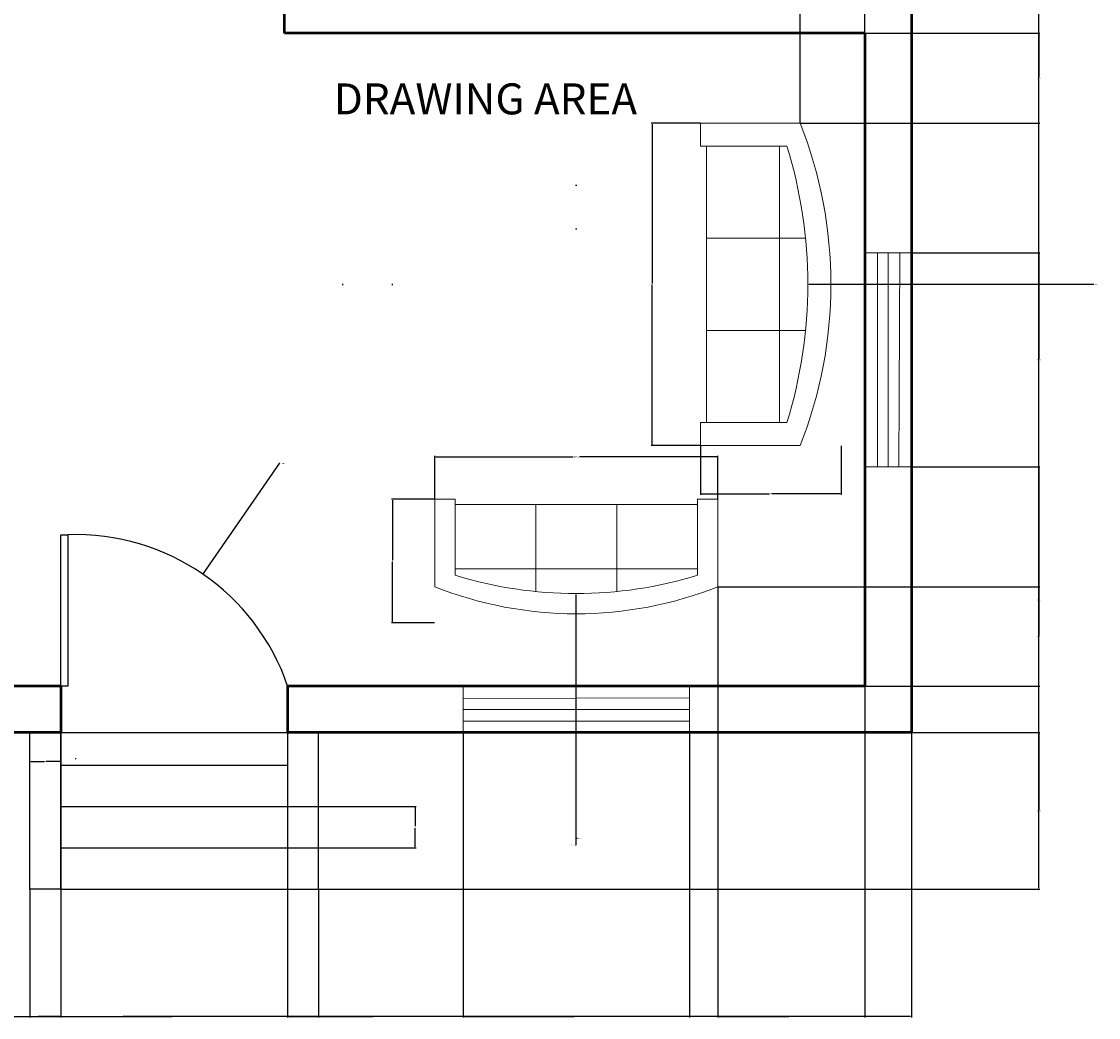
# Model space of a CAD drawing. Units: inches. Extents: x 1926 to 2293, y 1738 to 2280.
# Tile 2 of 6: x 2084 to 2293, y 1738 to 1931. Entities that reach past the tile are written whole.
import ezdxf

# ---------------------------------------------------------------- set-up
doc = ezdxf.new("R2010")
doc.units = ezdxf.units.IN
for name, color, linetype, lineweight in [('A-ANNO-DIMS', 2, 'Continuous', 18), ('A-AREA-IDEN', 7, 'Continuous', 25), ('A-DOOR', 3, 'Continuous', 25), ('A-FLOR-STRS', 7, 'Continuous', 25), ('A-FURN', 8, 'Continuous', 18), ('A-GLAZ', 4, 'Continuous', 18), ('A-WALL', 7, 'Continuous', 50)]:
    doc.layers.add(name, color=color, linetype=linetype, lineweight=lineweight)
doc.styles.get("Standard").update_dxf_attribs({"font": 'arial.ttf'})
doc.dimstyles.get("Standard").update_dxf_attribs({"dimtxt": 0.18, "dimasz": 0.18, "dimexe": 0.18, "dimexo": 0.0625, "dimgap": 0.09, "dimtad": 0, "dimtih": 1, "dimtoh": 1, "dimdec": 4, "dimzin": 0, "dimdsep": 46, "dimtxsty": 'Standard', "dimcen": 0.09, "dimadec": 0, "dimazin": 0, "dimtfac": 1, "dimtdec": 4, "dimtofl": 0, "dimtmove": 0, "dimatfit": 3, "dimfxl": 1, "dimtolj": 1, "dimtzin": 0, "dimarcsym": 0})

# ---------------------------------------------------------------- blocks, each defined once
blk = doc.blocks.new('Sofa - Roundback 7 ft.')
for p, q in [((-12.00002, -32.4421), (-12.00003, -6.5971)), ((11.99997, -32.4421), (11.99998, -6.5971)), ((-36.000027, -34), (-36.000027, -11.4696)), ((-35.999844, -13.3819), (35.9998, -13.3819)), ((35.99998, -34), (35.99998, -11.4696)), ((-36.000027, -32.4421), (35.99998, -32.4421))]:
    blk.add_line(p, q)
for points in [[(-36.000027, -34), (-42.000027, -34), (-42.000027, -8)], [(41.99998, -8), (41.99998, -34), (35.99998, -34)]]:
    blk.add_lwpolyline(points)
for centre, radius, start, end in [((0, -114.25), 114.25, 68.43141, 111.5686), ((-0.00001, -127.1968), 121.1968, 72.72033, 107.2797)]:
    blk.add_arc(centre, radius, start, end)
blk = doc.blocks.new('*D8')
at = {"layer": 'A-ANNO-DIMS', "color": 0, "lineweight": -2, "transparency": 16777216}
for p, q in [((2215.82, 1911.23), (2206.33, 1911.23)), ((2206.51, 1911.05), (2206.51, 1880.18)), ((2206.51, 1848.95), (2206.51, 1879.82)), ((2215.82, 1848.77), (2206.33, 1848.77))]:
    blk.add_line(p, q, dxfattribs=at)
at = {"layer": 'A-ANNO-DIMS', "color": 0, "transparency": 16777216}
for points in [[(2206.48, 1911.05), (2206.54, 1911.05), (2206.51, 1911.23)], [(2206.48, 1848.95), (2206.54, 1848.95), (2206.51, 1848.77)]]:
    blk.add_solid(points, dxfattribs=at)
at = {"layer": 'Defpoints', "color": 0, "transparency": 16777216}
for p in [(2215.88, 1911.23), (2206.51, 1848.77), (2215.88, 1848.77)]:
    blk.add_point(p, dxfattribs=at)
at = {"layer": 'A-ANNO-DIMS', "color": 0, "transparency": 16777216, "insert": (2206.51, 1880), "char_height": 0.18, "attachment_point": 5}
blk.add_mtext('\\A1;SOFA 62', dxfattribs=at)
blk = doc.blocks.new('*D9')
at = {"layer": 'A-ANNO-DIMS', "color": 0, "lineweight": -2, "transparency": 16777216}
for p, q in [((2215.88, 1848.71), (2215.88, 1839.22)), ((2243.14, 1848.71), (2243.14, 1839.22)), ((2216.06, 1839.4), (2229.29, 1839.4)), ((2242.96, 1839.4), (2229.73, 1839.4))]:
    blk.add_line(p, q, dxfattribs=at)
at = {"layer": 'A-ANNO-DIMS', "color": 0, "transparency": 16777216}
for points in [[(2216.06, 1839.43), (2216.06, 1839.37), (2215.88, 1839.4)], [(2242.96, 1839.43), (2242.96, 1839.37), (2243.14, 1839.4)]]:
    blk.add_solid(points, dxfattribs=at)
at = {"layer": 'Defpoints', "color": 0, "transparency": 16777216}
for p in [(2215.88, 1848.77), (2243.14, 1848.77), (2243.14, 1839.4)]:
    blk.add_point(p, dxfattribs=at)
at = {"layer": 'A-ANNO-DIMS', "color": 0, "transparency": 16777216, "insert": (2229.51, 1839.4), "char_height": 0.18, "attachment_point": 5}
blk.add_mtext('\\A1;27', dxfattribs=at)
blk = doc.blocks.new('*D10')
at = {"layer": 'A-ANNO-DIMS', "color": 0, "lineweight": -2, "transparency": 16777216}
for p, q in [((2164.42, 1838.43), (2164.42, 1846.77)), ((2164.6, 1846.59), (2191.24, 1846.59)), ((2219.07, 1846.59), (2192.43, 1846.59)), ((2219.25, 1838.43), (2219.25, 1846.77))]:
    blk.add_line(p, q, dxfattribs=at)
at = {"layer": 'A-ANNO-DIMS', "color": 0, "transparency": 16777216}
for points in [[(2164.6, 1846.62), (2164.6, 1846.56), (2164.42, 1846.59)], [(2219.07, 1846.62), (2219.07, 1846.56), (2219.25, 1846.59)]]:
    blk.add_solid(points, dxfattribs=at)
at = {"layer": 'Defpoints', "color": 0, "transparency": 16777216}
for p in [(2164.42, 1846.59), (2164.42, 1838.37), (2219.25, 1838.37)]:
    blk.add_point(p, dxfattribs=at)
at = {"layer": 'A-ANNO-DIMS', "color": 0, "transparency": 16777216, "insert": (2191.84, 1846.59), "char_height": 0.18, "attachment_point": 5}
blk.add_mtext('\\A1;SOFA 55', dxfattribs=at)
blk = doc.blocks.new('*D11')
at = {"layer": 'A-ANNO-DIMS', "color": 0, "lineweight": -2, "transparency": 16777216}
for p, q in [((2164.36, 1838.37), (2156.02, 1838.37)), ((2156.2, 1838.19), (2156.2, 1826.58)), ((2156.2, 1814.62), (2156.2, 1826.22)), ((2164.36, 1814.44), (2156.02, 1814.44))]:
    blk.add_line(p, q, dxfattribs=at)
at = {"layer": 'A-ANNO-DIMS', "color": 0, "transparency": 16777216}
for points in [[(2156.17, 1838.19), (2156.23, 1838.19), (2156.2, 1838.37)], [(2156.17, 1814.62), (2156.23, 1814.62), (2156.2, 1814.44)]]:
    blk.add_solid(points, dxfattribs=at)
at = {"layer": 'Defpoints', "color": 0, "transparency": 16777216}
for p in [(2164.42, 1838.37), (2156.2, 1814.44), (2164.42, 1814.44)]:
    blk.add_point(p, dxfattribs=at)
at = {"layer": 'A-ANNO-DIMS', "color": 0, "transparency": 16777216, "insert": (2156.2, 1826.4), "char_height": 0.18, "attachment_point": 5}
blk.add_mtext('\\A1;24', dxfattribs=at)
blk = doc.blocks.new('*D28')
at = {"layer": 'A-ANNO-DIMS', "color": 0, "lineweight": -2, "transparency": 16777216}
for p, q in [((2082.76, 1802.1), (2082.76, 1737.97)), ((2091.96, 1802.1), (2091.96, 1737.97)), ((2082.94, 1738.15), (2087.1, 1738.15)), ((2091.78, 1738.15), (2087.61, 1738.15))]:
    blk.add_line(p, q, dxfattribs=at)
at = {"layer": 'A-ANNO-DIMS', "color": 0, "transparency": 16777216}
for points in [[(2082.94, 1738.18), (2082.94, 1738.12), (2082.76, 1738.15)], [(2091.78, 1738.18), (2091.78, 1738.12), (2091.96, 1738.15)]]:
    blk.add_solid(points, dxfattribs=at)
at = {"layer": 'Defpoints', "color": 0, "transparency": 16777216}
for p in [(2082.76, 1802.16), (2091.96, 1802.16), (2091.96, 1738.15)]:
    blk.add_point(p, dxfattribs=at)
at = {"layer": 'A-ANNO-DIMS', "color": 0, "transparency": 16777216, "insert": (2087.36, 1738.15), "char_height": 0.18, "attachment_point": 5}
blk.add_mtext('\\A1;9.2', dxfattribs=at)
blk = doc.blocks.new('*D29')
at = {"layer": 'A-ANNO-DIMS', "color": 0, "lineweight": -2, "transparency": 16777216}
for p, q in [((2091.96, 1793.1), (2091.96, 1737.97)), ((2135.91, 1793.1), (2135.91, 1737.97)), ((2092.14, 1738.15), (2113.54, 1738.15)), ((2135.73, 1738.15), (2114.33, 1738.15))]:
    blk.add_line(p, q, dxfattribs=at)
at = {"layer": 'A-ANNO-DIMS', "color": 0, "transparency": 16777216}
for points in [[(2092.14, 1738.18), (2092.14, 1738.12), (2091.96, 1738.15)], [(2135.73, 1738.18), (2135.73, 1738.12), (2135.91, 1738.15)]]:
    blk.add_solid(points, dxfattribs=at)
at = {"layer": 'Defpoints', "color": 0, "transparency": 16777216}
for p in [(2091.96, 1793.16), (2135.91, 1793.16), (2135.91, 1738.15)]:
    blk.add_point(p, dxfattribs=at)
at = {"layer": 'A-ANNO-DIMS', "color": 0, "transparency": 16777216, "insert": (2113.94, 1738.15), "char_height": 0.18, "attachment_point": 5}
blk.add_mtext('\\A1;43.96', dxfattribs=at)
blk = doc.blocks.new('*D30')
at = {"layer": 'A-ANNO-DIMS', "color": 0, "lineweight": -2, "transparency": 16777216}
for p, q in [((2135.91, 1793.1), (2135.91, 1737.97)), ((2169.91, 1793.1), (2169.91, 1737.97)), ((2136.09, 1738.15), (2152.45, 1738.15)), ((2169.73, 1738.15), (2153.37, 1738.15))]:
    blk.add_line(p, q, dxfattribs=at)
at = {"layer": 'A-ANNO-DIMS', "color": 0, "transparency": 16777216}
for points in [[(2136.09, 1738.18), (2136.09, 1738.12), (2135.91, 1738.15)], [(2169.73, 1738.18), (2169.73, 1738.12), (2169.91, 1738.15)]]:
    blk.add_solid(points, dxfattribs=at)
at = {"layer": 'Defpoints', "color": 0, "transparency": 16777216}
for p in [(2135.91, 1793.16), (2169.91, 1793.16), (2169.91, 1738.15)]:
    blk.add_point(p, dxfattribs=at)
at = {"layer": 'A-ANNO-DIMS', "color": 0, "transparency": 16777216, "insert": (2152.91, 1738.15), "char_height": 0.18, "attachment_point": 5}
blk.add_mtext('\\A1;33.994', dxfattribs=at)
blk = doc.blocks.new('*D31')
at = {"layer": 'A-ANNO-DIMS', "color": 0, "lineweight": -2, "transparency": 16777216}
for p, q in [((2169.91, 1793.1), (2169.91, 1737.97)), ((2213.78, 1793.1), (2213.78, 1737.97)), ((2170.09, 1738.15), (2191.45, 1738.15)), ((2213.6, 1738.15), (2192.24, 1738.15))]:
    blk.add_line(p, q, dxfattribs=at)
at = {"layer": 'A-ANNO-DIMS', "color": 0, "transparency": 16777216}
for points in [[(2170.09, 1738.18), (2170.09, 1738.12), (2169.91, 1738.15)], [(2213.6, 1738.18), (2213.6, 1738.12), (2213.78, 1738.15)]]:
    blk.add_solid(points, dxfattribs=at)
at = {"layer": 'Defpoints', "color": 0, "transparency": 16777216}
for p in [(2169.91, 1793.16), (2213.78, 1793.16), (2213.78, 1738.15)]:
    blk.add_point(p, dxfattribs=at)
at = {"layer": 'A-ANNO-DIMS', "color": 0, "transparency": 16777216, "insert": (2191.84, 1738.15), "char_height": 0.18, "attachment_point": 5}
blk.add_mtext('\\A1;43.87', dxfattribs=at)
blk = doc.blocks.new('*D32')
at = {"layer": 'A-ANNO-DIMS', "color": 0, "lineweight": -2, "transparency": 16777216}
for p, q in [((2085.96, 1762.79), (2085.96, 1737.97)), ((2141.91, 1762.79), (2141.91, 1737.97)), ((2086.14, 1738.15), (2113.54, 1738.15)), ((2141.73, 1738.15), (2114.33, 1738.15))]:
    blk.add_line(p, q, dxfattribs=at)
at = {"layer": 'A-ANNO-DIMS', "color": 0, "transparency": 16777216}
for points in [[(2086.14, 1738.18), (2086.14, 1738.12), (2085.96, 1738.15)], [(2141.73, 1738.18), (2141.73, 1738.12), (2141.91, 1738.15)]]:
    blk.add_solid(points, dxfattribs=at)
at = {"layer": 'Defpoints', "color": 0, "transparency": 16777216}
for p in [(2085.96, 1762.85), (2141.91, 1762.85), (2141.91, 1738.15)]:
    blk.add_point(p, dxfattribs=at)
at = {"layer": 'A-ANNO-DIMS', "color": 0, "transparency": 16777216, "insert": (2113.94, 1738.15), "char_height": 0.18, "attachment_point": 5}
blk.add_mtext('\\A1;55.96', dxfattribs=at)
blk = doc.blocks.new('*D33')
at = {"layer": 'A-ANNO-DIMS', "color": 0, "lineweight": -2, "transparency": 16777216}
for p, q in [((2085.96, 1762.91), (2085.96, 1787.73)), ((2086.14, 1787.55), (2088.81, 1787.55)), ((2091.78, 1787.55), (2089.11, 1787.55)), ((2091.96, 1762.91), (2091.96, 1787.73))]:
    blk.add_line(p, q, dxfattribs=at)
at = {"layer": 'A-ANNO-DIMS', "color": 0, "transparency": 16777216}
for points in [[(2086.14, 1787.58), (2086.14, 1787.52), (2085.96, 1787.55)], [(2091.78, 1787.58), (2091.78, 1787.52), (2091.96, 1787.55)]]:
    blk.add_solid(points, dxfattribs=at)
at = {"layer": 'Defpoints', "color": 0, "transparency": 16777216}
for p in [(2091.96, 1787.55), (2085.96, 1762.85), (2091.96, 1762.85)]:
    blk.add_point(p, dxfattribs=at)
at = {"layer": 'A-ANNO-DIMS', "color": 0, "transparency": 16777216, "insert": (2088.96, 1787.55), "char_height": 0.18, "attachment_point": 5}
blk.add_mtext('\\A1;6', dxfattribs=at)
blk = doc.blocks.new('*D34')
at = {"layer": 'A-ANNO-DIMS', "color": 0, "lineweight": -2, "transparency": 16777216}
for p, q in [((2135.98, 1778.85), (2160.79, 1778.85)), ((2160.61, 1778.67), (2160.61, 1775.03)), ((2160.61, 1771.03), (2160.61, 1774.67)), ((2135.98, 1770.85), (2160.79, 1770.85))]:
    blk.add_line(p, q, dxfattribs=at)
at = {"layer": 'A-ANNO-DIMS', "color": 0, "transparency": 16777216}
for points in [[(2160.58, 1778.67), (2160.64, 1778.67), (2160.61, 1778.85)], [(2160.58, 1771.03), (2160.64, 1771.03), (2160.61, 1770.85)]]:
    blk.add_solid(points, dxfattribs=at)
at = {"layer": 'Defpoints', "color": 0, "transparency": 16777216}
for p in [(2135.91, 1778.85), (2135.91, 1770.85), (2160.61, 1770.85)]:
    blk.add_point(p, dxfattribs=at)
at = {"layer": 'A-ANNO-DIMS', "color": 0, "transparency": 16777216, "insert": (2160.61, 1774.85), "char_height": 0.18, "attachment_point": 5}
blk.add_mtext('\\A1;8', dxfattribs=at)
blk = doc.blocks.new('*D35')
at = {"layer": 'A-ANNO-DIMS', "color": 0, "lineweight": -2, "transparency": 16777216}
for p, q in [((2141.98, 1793.16), (2281.64, 1793.16)), ((2281.46, 1792.98), (2281.46, 1778.19)), ((2281.46, 1763.03), (2281.46, 1777.83)), ((2141.98, 1762.85), (2281.64, 1762.85))]:
    blk.add_line(p, q, dxfattribs=at)
at = {"layer": 'A-ANNO-DIMS', "color": 0, "transparency": 16777216}
for points in [[(2281.43, 1792.98), (2281.49, 1792.98), (2281.46, 1793.16)], [(2281.43, 1763.03), (2281.49, 1763.03), (2281.46, 1762.85)]]:
    blk.add_solid(points, dxfattribs=at)
at = {"layer": 'Defpoints', "color": 0, "transparency": 16777216}
for p in [(2141.91, 1793.16), (2281.46, 1793.16), (2141.91, 1762.85)]:
    blk.add_point(p, dxfattribs=at)
at = {"layer": 'A-ANNO-DIMS', "color": 0, "transparency": 16777216, "insert": (2281.46, 1778.01), "char_height": 0.18, "attachment_point": 5}
blk.add_mtext('\\A1;30.31', dxfattribs=at)
blk = doc.blocks.new('*D42')
at = {"layer": 'A-ANNO-DIMS', "color": 0, "lineweight": -2, "transparency": 16777216}
for p, q in [((2256.82, 1844.62), (2281.64, 1844.62)), ((2281.46, 1844.44), (2281.46, 1819.07)), ((2281.46, 1793.34), (2281.46, 1818.71)), ((2256.82, 1793.16), (2281.64, 1793.16))]:
    blk.add_line(p, q, dxfattribs=at)
at = {"layer": 'A-ANNO-DIMS', "color": 0, "transparency": 16777216}
for points in [[(2281.43, 1844.44), (2281.49, 1844.44), (2281.46, 1844.62)], [(2281.43, 1793.34), (2281.49, 1793.34), (2281.46, 1793.16)]]:
    blk.add_solid(points, dxfattribs=at)
at = {"layer": 'Defpoints', "color": 0, "transparency": 16777216}
for p in [(2256.76, 1844.62), (2281.46, 1844.62), (2256.76, 1793.16)]:
    blk.add_point(p, dxfattribs=at)
at = {"layer": 'A-ANNO-DIMS', "color": 0, "transparency": 16777216, "insert": (2281.46, 1818.89), "char_height": 0.18, "attachment_point": 5}
blk.add_mtext('\\A1;51.46', dxfattribs=at)
blk = doc.blocks.new('*D43')
at = {"layer": 'A-ANNO-DIMS', "color": 0, "lineweight": -2, "transparency": 16777216}
for p, q in [((2256.82, 1886.13), (2281.64, 1886.13)), ((2281.46, 1885.95), (2281.46, 1865.56)), ((2281.46, 1844.8), (2281.46, 1865.19)), ((2256.82, 1844.62), (2281.64, 1844.62))]:
    blk.add_line(p, q, dxfattribs=at)
at = {"layer": 'A-ANNO-DIMS', "color": 0, "transparency": 16777216}
for points in [[(2281.43, 1885.95), (2281.49, 1885.95), (2281.46, 1886.13)], [(2281.43, 1844.8), (2281.49, 1844.8), (2281.46, 1844.62)]]:
    blk.add_solid(points, dxfattribs=at)
at = {"layer": 'Defpoints', "color": 0, "transparency": 16777216}
for p in [(2256.76, 1886.13), (2281.46, 1886.13), (2256.76, 1844.62)]:
    blk.add_point(p, dxfattribs=at)
at = {"layer": 'A-ANNO-DIMS', "color": 0, "transparency": 16777216, "insert": (2281.46, 1865.37), "char_height": 0.18, "attachment_point": 5}
blk.add_mtext('\\A1;41.51', dxfattribs=at)
blk = doc.blocks.new('*D71')
at = {"layer": 'A-ANNO-DIMS', "color": 0, "lineweight": -2, "transparency": 16777216}
for p, q in [((2247.82, 1928.66), (2281.64, 1928.66)), ((2281.46, 1928.48), (2281.46, 1920.13)), ((2281.46, 1911.41), (2281.46, 1919.76)), ((2235.27, 1911.23), (2281.64, 1911.23))]:
    blk.add_line(p, q, dxfattribs=at)
at = {"layer": 'A-ANNO-DIMS', "color": 0, "transparency": 16777216}
for points in [[(2281.43, 1928.48), (2281.49, 1928.48), (2281.46, 1928.66)], [(2281.43, 1911.41), (2281.49, 1911.41), (2281.46, 1911.23)]]:
    blk.add_solid(points, dxfattribs=at)
at = {"layer": 'Defpoints', "color": 0, "transparency": 16777216}
for p in [(2247.76, 1928.66), (2281.46, 1928.66), (2235.21, 1911.23)]:
    blk.add_point(p, dxfattribs=at)
at = {"layer": 'A-ANNO-DIMS', "color": 0, "transparency": 16777216, "insert": (2281.46, 1919.95), "char_height": 0.18, "attachment_point": 5}
blk.add_mtext('\\A1;17.43', dxfattribs=at)
blk = doc.blocks.new('*D72')
at = {"layer": 'A-ANNO-DIMS', "color": 0, "lineweight": -2, "transparency": 16777216}
for p, q in [((2235.21, 1911.29), (2235.21, 2280.04)), ((2235.39, 2279.86), (2241.03, 2279.86)), ((2247.58, 2279.86), (2241.94, 2279.86)), ((2247.76, 1928.72), (2247.76, 2280.04))]:
    blk.add_line(p, q, dxfattribs=at)
at = {"layer": 'A-ANNO-DIMS', "color": 0, "transparency": 16777216}
for points in [[(2235.39, 2279.89), (2235.39, 2279.83), (2235.21, 2279.86)], [(2247.58, 2279.89), (2247.58, 2279.83), (2247.76, 2279.86)]]:
    blk.add_solid(points, dxfattribs=at)
at = {"layer": 'Defpoints', "color": 0, "transparency": 16777216}
for p in [(2247.76, 2279.86), (2247.76, 1928.66), (2235.21, 1911.23)]:
    blk.add_point(p, dxfattribs=at)
at = {"layer": 'A-ANNO-DIMS', "color": 0, "transparency": 16777216, "insert": (2241.48, 2279.86), "char_height": 0.18, "attachment_point": 5}
blk.add_mtext('\\A1;12.546', dxfattribs=at)
blk = doc.blocks.new('*D73')
at = {"layer": 'A-ANNO-DIMS', "color": 0, "lineweight": -2, "transparency": 16777216}
for p, q in [((2219.32, 1821.4), (2281.64, 1821.4)), ((2281.46, 1821.22), (2281.46, 1811.96)), ((2281.46, 1802.34), (2281.46, 1811.6)), ((2247.82, 1802.16), (2281.64, 1802.16))]:
    blk.add_line(p, q, dxfattribs=at)
at = {"layer": 'A-ANNO-DIMS', "color": 0, "transparency": 16777216}
for points in [[(2281.43, 1821.22), (2281.49, 1821.22), (2281.46, 1821.4)], [(2281.43, 1802.34), (2281.49, 1802.34), (2281.46, 1802.16)]]:
    blk.add_solid(points, dxfattribs=at)
at = {"layer": 'Defpoints', "color": 0, "transparency": 16777216}
for p in [(2219.25, 1821.4), (2247.76, 1802.16), (2281.46, 1802.16)]:
    blk.add_point(p, dxfattribs=at)
at = {"layer": 'A-ANNO-DIMS', "color": 0, "transparency": 16777216, "insert": (2281.46, 1811.78), "char_height": 0.18, "attachment_point": 5}
blk.add_mtext('\\A1;19.236', dxfattribs=at)
blk = doc.blocks.new('*D74')
at = {"layer": 'A-ANNO-DIMS', "color": 0, "lineweight": -2, "transparency": 16777216}
for p, q in [((2219.25, 1821.34), (2219.25, 1737.97)), ((2247.76, 1802.1), (2247.76, 1737.97)), ((2219.43, 1738.15), (2233.04, 1738.15)), ((2247.58, 1738.15), (2233.97, 1738.15))]:
    blk.add_line(p, q, dxfattribs=at)
at = {"layer": 'A-ANNO-DIMS', "color": 0, "transparency": 16777216}
for points in [[(2219.43, 1738.18), (2219.43, 1738.12), (2219.25, 1738.15)], [(2247.58, 1738.18), (2247.58, 1738.12), (2247.76, 1738.15)]]:
    blk.add_solid(points, dxfattribs=at)
at = {"layer": 'Defpoints', "color": 0, "transparency": 16777216}
for p in [(2219.25, 1821.4), (2247.76, 1802.16), (2247.76, 1738.15)]:
    blk.add_point(p, dxfattribs=at)
at = {"layer": 'A-ANNO-DIMS', "color": 0, "transparency": 16777216, "insert": (2233.51, 1738.15), "char_height": 0.18, "attachment_point": 5}
blk.add_mtext('\\A1;28.503', dxfattribs=at)
blk = doc.blocks.new('*D84')
at = {"layer": 'A-ANNO-DIMS', "color": 0, "lineweight": -2, "transparency": 16777216}
for p, q in [((1950.76, 1793.1), (1950.76, 1737.97)), ((2256.76, 1793.1), (2256.76, 1737.97)), ((1950.94, 1738.15), (2103.47, 1738.15)), ((2256.58, 1738.15), (2104.05, 1738.15))]:
    blk.add_line(p, q, dxfattribs=at)
at = {"layer": 'A-ANNO-DIMS', "color": 0, "transparency": 16777216}
for points in [[(1950.94, 1738.18), (1950.94, 1738.12), (1950.76, 1738.15)], [(2256.58, 1738.18), (2256.58, 1738.12), (2256.76, 1738.15)]]:
    blk.add_solid(points, dxfattribs=at)
at = {"layer": 'Defpoints', "color": 0, "transparency": 16777216}
for p in [(1950.76, 1793.16), (2256.76, 1793.16), (2256.76, 1738.15)]:
    blk.add_point(p, dxfattribs=at)
at = {"layer": 'A-ANNO-DIMS', "color": 0, "transparency": 16777216, "insert": (2103.76, 1738.15), "char_height": 0.18, "attachment_point": 5}
blk.add_mtext('\\A1;306', dxfattribs=at)
blk = doc.blocks.new('*D86')
at = {"layer": 'A-ANNO-DIMS', "color": 0, "lineweight": -2, "transparency": 16777216}
for p, q in [((2256.82, 2255.16), (2281.64, 2255.16)), ((2281.46, 2254.98), (2281.46, 2009.19)), ((2281.46, 1763.03), (2281.46, 2008.83)), ((2141.98, 1762.85), (2281.64, 1762.85))]:
    blk.add_line(p, q, dxfattribs=at)
at = {"layer": 'A-ANNO-DIMS', "color": 0, "transparency": 16777216}
for points in [[(2281.43, 2254.98), (2281.49, 2254.98), (2281.46, 2255.16)], [(2281.43, 1763.03), (2281.49, 1763.03), (2281.46, 1762.85)]]:
    blk.add_solid(points, dxfattribs=at)
at = {"layer": 'Defpoints', "color": 0, "transparency": 16777216}
for p in [(2256.76, 2255.16), (2281.46, 2255.16), (2141.91, 1762.85)]:
    blk.add_point(p, dxfattribs=at)
at = {"layer": 'A-ANNO-DIMS', "color": 0, "transparency": 16777216, "insert": (2281.46, 2009.01), "char_height": 0.18, "attachment_point": 5}
blk.add_mtext('\\A1;492.3', dxfattribs=at)
blk = doc.blocks.new('*D87')
at = {"layer": 'A-ANNO-DIMS', "color": 0, "lineweight": -2, "transparency": 16777216}
for p, q in [((2134.24, 1845.3), (2119.57, 1824.01)), ((2134.42, 1845.3), (2134.24, 1845.3)), ((2094.77, 1788.14), (2094.95, 1788.14)), ((2094.86, 1788.05), (2094.86, 1788.23))]:
    blk.add_line(p, q, dxfattribs=at)
at = {"layer": 'A-ANNO-DIMS', "color": 0, "transparency": 16777216}
blk.add_solid([(2119.55, 1824.03), (2119.6, 1824), (2119.47, 1823.86)], dxfattribs=at)
at = {"layer": 'Defpoints', "color": 0, "transparency": 16777216}
for p in [(2119.47, 1823.86), (2094.86, 1788.14)]:
    blk.add_point(p, dxfattribs=at)
at = {"layer": 'A-ANNO-DIMS', "color": 0, "transparency": 16777216, "insert": (2134.9, 1845.3), "char_height": 0.18, "attachment_point": 5}
blk.add_mtext('\\A1;R43.38', dxfattribs=at)
blk = doc.blocks.new('*D103')
at = {"layer": 'A-ANNO-DIMS', "color": 0, "lineweight": -2, "transparency": 16777216}
for p, q in [((2146.49, 1880), (2146.67, 1880)), ((2146.58, 1879.91), (2146.58, 1880.09)), ((2290.77, 1880), (2236.88, 1880))]:
    blk.add_line(p, q, dxfattribs=at)
at = {"layer": 'A-ANNO-DIMS', "color": 0, "transparency": 16777216}
blk.add_solid([(2236.88, 1880.03), (2236.88, 1879.97), (2236.7, 1880)], dxfattribs=at)
at = {"layer": 'Defpoints', "color": 0, "transparency": 16777216}
for p in [(2146.58, 1880), (2236.7, 1880)]:
    blk.add_point(p, dxfattribs=at)
at = {"layer": 'A-ANNO-DIMS', "color": 0, "transparency": 16777216, "insert": (2291.25, 1880), "char_height": 0.18, "attachment_point": 5}
blk.add_mtext('\\A1;R90.12', dxfattribs=at)
blk = doc.blocks.new('*D104')
at = {"layer": 'A-ANNO-DIMS', "color": 0, "lineweight": -2, "transparency": 16777216}
for p, q in [((2156.12, 1880), (2156.3, 1880)), ((2156.21, 1879.91), (2156.21, 1880.09)), ((2292.13, 1880), (2241.34, 1880))]:
    blk.add_line(p, q, dxfattribs=at)
at = {"layer": 'A-ANNO-DIMS', "color": 0, "transparency": 16777216}
blk.add_solid([(2241.34, 1880.03), (2241.34, 1879.97), (2241.16, 1880)], dxfattribs=at)
at = {"layer": 'Defpoints', "color": 0, "transparency": 16777216}
for p in [(2156.21, 1880), (2241.16, 1880)]:
    blk.add_point(p, dxfattribs=at)
at = {"layer": 'A-ANNO-DIMS', "color": 0, "transparency": 16777216, "insert": (2292.61, 1880), "char_height": 0.18, "attachment_point": 5}
blk.add_mtext('\\A1;R84.95', dxfattribs=at)
blk = doc.blocks.new('*D105')
at = {"layer": 'A-ANNO-DIMS', "color": 0, "lineweight": -2, "transparency": 16777216}
for p, q in [((2191.75, 1899.2), (2191.93, 1899.2)), ((2191.84, 1899.11), (2191.84, 1899.29)), ((2191.84, 1772.63), (2191.84, 1819.91)), ((2192.02, 1772.63), (2191.84, 1772.63))]:
    blk.add_line(p, q, dxfattribs=at)
at = {"layer": 'A-ANNO-DIMS', "color": 0, "transparency": 16777216}
blk.add_solid([(2191.87, 1819.91), (2191.81, 1819.91), (2191.84, 1820.09)], dxfattribs=at)
at = {"layer": 'Defpoints', "color": 0, "transparency": 16777216}
for p in [(2191.84, 1899.2), (2191.84, 1820.09)]:
    blk.add_point(p, dxfattribs=at)
at = {"layer": 'A-ANNO-DIMS', "color": 0, "transparency": 16777216, "insert": (2192.48, 1772.63), "char_height": 0.18, "attachment_point": 5}
blk.add_mtext('\\A1;R79.11', dxfattribs=at)
blk = doc.blocks.new('*D106')
at = {"layer": 'A-ANNO-DIMS', "color": 0, "lineweight": -2, "transparency": 16777216}
for p, q in [((2191.75, 1890.75), (2191.93, 1890.75)), ((2191.84, 1890.66), (2191.84, 1890.84)), ((2191.84, 1771.43), (2191.84, 1816)), ((2191.66, 1771.43), (2191.84, 1771.43))]:
    blk.add_line(p, q, dxfattribs=at)
at = {"layer": 'A-ANNO-DIMS', "color": 0, "transparency": 16777216}
blk.add_solid([(2191.81, 1816), (2191.87, 1816), (2191.84, 1816.18)], dxfattribs=at)
at = {"layer": 'Defpoints', "color": 0, "transparency": 16777216}
for p in [(2191.84, 1890.75), (2191.84, 1816.18)]:
    blk.add_point(p, dxfattribs=at)
at = {"layer": 'A-ANNO-DIMS', "color": 0, "transparency": 16777216, "insert": (2191.18, 1771.43), "char_height": 0.18, "attachment_point": 5}
blk.add_mtext('\\A1;R74.58', dxfattribs=at)

msp = doc.modelspace()

# ---------------------------------------------------------------- linework, layer by layer
at = {"layer": 'A-DOOR'}
for p, q in [((2091.9575, 1802.1622), (2091.9575, 1831.4942)), ((2091.9575, 1831.4942), (2093.3367, 1831.4942)), ((2093.3367, 1831.4942), (2093.3367, 1802.1622)), ((2093.3367, 1802.1622), (2091.9575, 1802.1622))]:
    msp.add_line(p, q, dxfattribs=at)
msp.add_arc((2094.863, 1788.1407), 43.3803, 18.857933, 92.016262, dxfattribs=at)
at = {"layer": 'A-FLOR-STRS'}
for p, q in [((2085.9575, 1762.8524), (2085.9575, 1793.1622)), ((2091.9575, 1793.1622), (2135.9148, 1793.1622)), ((2091.9575, 1762.8524), (2091.9575, 1793.1622)), ((2135.9148, 1793.1622), (2135.9148, 1762.8524)), ((2141.9148, 1762.8524), (2141.9148, 1793.1622)), ((2091.9575, 1786.8524), (2135.9148, 1786.8524)), ((2091.9575, 1778.8524), (2135.9148, 1778.8524)), ((2091.9575, 1770.8524), (2135.9148, 1770.8524)), ((2091.9575, 1762.8524), (2085.9575, 1762.8524)), ((2091.9575, 1762.8524), (2135.9148, 1762.8524)), ((2135.9148, 1762.8524), (2141.9148, 1762.8524))]:
    msp.add_line(p, q, dxfattribs=at)
at = {"layer": 'A-GLAZ'}
for p, q in [((2250.1729, 1886.1313), (2250.1729, 1844.618)), ((2252.2569, 1886.1313), (2252.2569, 1844.618)), ((2254.5273, 1886.1313), (2254.342, 1844.618)), ((2169.9087, 1799.7795), (2213.7782, 1799.8947)), ((2169.9087, 1797.6622), (2213.7782, 1797.6622)), ((2169.9087, 1795.3422), (2213.7782, 1795.3422))]:
    msp.add_line(p, q, dxfattribs=at)
for points in [[(2247.7569, 1886.1313), (2256.7569, 1886.1313), (2256.7569, 1844.618), (2247.7569, 1844.618)], [(2169.9087, 1802.1622), (2213.7782, 1802.1622), (2213.7782, 1793.1622), (2169.9087, 1793.1622)]]:
    msp.add_lwpolyline(points, close=True, dxfattribs=at)
at = {"layer": 'A-WALL'}
for p, q in [((2256.7569, 2255.1622), (2256.7569, 1793.1622)), ((2135.2979, 1928.6622), (2135.2979, 1933.1622)), ((2247.7569, 1928.6622), (2135.2979, 1928.6622)), ((2247.7569, 1928.6622), (2247.7569, 1802.1622)), ((2091.9575, 1802.1622), (2082.7569, 1802.1622)), ((2091.9575, 1802.1622), (2091.9575, 1793.1622)), ((2247.7569, 1802.1622), (2135.9148, 1802.1622)), ((2135.9148, 1802.1622), (2135.9148, 1793.1622)), ((2091.9575, 1793.1622), (1950.7569, 1793.1622)), ((2256.7569, 1793.1622), (2135.9148, 1793.1622))]:
    msp.add_line(p, q, dxfattribs=at)

# ---------------------------------------------------------------- block references
at = {"layer": 'A-FURN'}
for p, xscale, yscale, zscale, rotation in [((2241.1598, 1880.0003), 0.7435785128575735, 0.7435785128575735, 0.7435785128575735, 270), ((2191.8385, 1816.1762), 0.6527429926504595, 0.6527429926504595, 0.6527429926504595, 180)]:
    msp.add_blockref('Sofa - Roundback 7 ft.', p, dxfattribs=dict(at, xscale=xscale, yscale=yscale, zscale=zscale, rotation=rotation))

# ---------------------------------------------------------------- texts
at = {"layer": 'A-AREA-IDEN', "insert": (2144.8524, 1918.9282), "char_height": 6, "attachment_point": 1}
msp.add_mtext_dynamic_manual_height_columns('DRAWING AREA', width=66.90772, gutter_width=12.5, heights=[0], dxfattribs=at)

# ---------------------------------------------------------------- dimensions: what is measured, and where the dimension line sits
at = {"layer": 'A-ANNO-DIMS'}
for base, p1, p2, override, picture, middle in [((2247.7569, 2279.8622), (2235.2111, 1911.2306), (2247.7569, 1928.6622), {"dimdec": 3, "dimlfac": 1, "dimrnd": 0, "dimzin": 0, "dimdsep": 46, "dimlunit": 2}, '*D72', (2241.484, 2279.8622)), ((2243.1426, 1839.4009), (2215.8781, 1848.77), (2243.1426, 1848.77), {"dimdec": 0, "dimlfac": 1, "dimrnd": 0, "dimzin": 0, "dimdsep": 46, "dimlunit": 2}, '*D9', (2229.5104, 1839.4009)), ((2247.7569, 1738.1524), (2219.2537, 1821.3982), (2247.7569, 1802.1622), {"dimdec": 3, "dimlfac": 1, "dimrnd": 0, "dimzin": 0, "dimdsep": 46, "dimlunit": 2}, '*D74', (2233.5053, 1738.1524)), ((2091.9575, 1738.1524), (2082.7569, 1802.1622), (2091.9575, 1802.1622), {"dimdec": 1, "dimlfac": 1, "dimrnd": 0, "dimzin": 0, "dimdsep": 46, "dimlunit": 2}, '*D28', (2087.3572, 1738.1524)), ((2256.7569, 1738.1524), (1950.7569, 1793.1622), (2256.7569, 1793.1622), {"dimdec": 0, "dimlfac": 1, "dimrnd": 0, "dimzin": 0, "dimdsep": 46, "dimlunit": 2}, '*D84', (2103.7569, 1738.1524)), ((2135.9148, 1738.1524), (2091.9575, 1793.1622), (2135.9148, 1793.1622), {"dimdec": 2, "dimlfac": 1, "dimrnd": 0, "dimzin": 0, "dimdsep": 46, "dimlunit": 2}, '*D29', (2113.9361, 1738.1524)), ((2169.9087, 1738.1524), (2135.9148, 1793.1622), (2169.9087, 1793.1622), {"dimdec": 3, "dimlfac": 1, "dimrnd": 0, "dimzin": 0, "dimdsep": 46, "dimlunit": 2}, '*D30', (2152.9117, 1738.1524)), ((2213.7782, 1738.1524), (2169.9087, 1793.1622), (2213.7782, 1793.1622), {"dimdec": 2, "dimlfac": 1, "dimrnd": 0, "dimzin": 0, "dimdsep": 46, "dimlunit": 2}, '*D31', (2191.8434, 1738.1524)), ((2091.9575, 1787.5524), (2085.9575, 1762.8524), (2091.9575, 1762.8524), {"dimdec": 0, "dimlfac": 1, "dimrnd": 0, "dimzin": 0, "dimdsep": 46, "dimlunit": 2}, '*D33', (2088.9575, 1787.5524)), ((2141.9148, 1738.1524), (2085.9575, 1762.8524), (2141.9148, 1762.8524), {"dimdec": 2, "dimlfac": 1, "dimrnd": 0, "dimzin": 0, "dimdsep": 46, "dimlunit": 2}, '*D32', (2113.9361, 1738.1524))]:
    dim = msp.add_linear_dim(base=base, p1=p1, p2=p2, dimstyle='Standard', override=override, dxfattribs=at)
    dim.commit()
    dim.dimension.update_dxf_attribs({"geometry": picture, "text_midpoint": middle})
for base, p1, p2, angle, override, picture, middle in [((2281.4569, 2255.1622), (2141.9148, 1762.8524), (2256.7569, 2255.1622), 90, {"dimdec": 1, "dimlfac": 1, "dimrnd": 0, "dimzin": 0, "dimdsep": 46, "dimlunit": 2}, '*D86', (2281.4569, 2009.0073)), ((2281.4569, 1928.6622), (2235.2111, 1911.2306), (2247.7569, 1928.6622), 90, {"dimdec": 2, "dimlfac": 1, "dimrnd": 0, "dimzin": 0, "dimdsep": 46, "dimlunit": 2}, '*D71', (2281.4569, 1919.9464)), ((2281.4569, 1886.1313), (2256.7569, 1844.618), (2256.7569, 1886.1313), 90, {"dimdec": 2, "dimlfac": 1, "dimrnd": 0, "dimzin": 0, "dimdsep": 46, "dimlunit": 2}, '*D43', (2281.4569, 1865.3746)), ((2281.4569, 1844.618), (2256.7569, 1793.1622), (2256.7569, 1844.618), 90, {"dimdec": 2, "dimlfac": 1, "dimrnd": 0, "dimzin": 0, "dimdsep": 46, "dimlunit": 2}, '*D42', (2281.4569, 1818.8901)), ((2156.1987, 1814.4356), (2164.4233, 1838.3695), (2164.4233, 1814.4356), 270, {"dimdec": 0, "dimlfac": 1, "dimrnd": 0, "dimzin": 0, "dimdsep": 46, "dimlunit": 2}, '*D11', (2156.1987, 1826.4025)), ((2281.4569, 1802.1622), (2219.2537, 1821.3982), (2247.7569, 1802.1622), 90, {"dimdec": 3, "dimlfac": 1, "dimrnd": 0, "dimzin": 0, "dimdsep": 46, "dimlunit": 2}, '*D73', (2281.4569, 1811.7802)), ((2281.4569, 1793.1622), (2141.9148, 1762.8524), (2141.9148, 1793.1622), 90, {"dimdec": 2, "dimlfac": 1, "dimrnd": 0, "dimzin": 0, "dimdsep": 46, "dimlunit": 2}, '*D35', (2281.4569, 1778.0073)), ((2160.6148, 1770.8524), (2135.9148, 1778.8524), (2135.9148, 1770.8524), 270, {"dimdec": 0, "dimlfac": 1, "dimrnd": 0, "dimzin": 0, "dimdsep": 46, "dimlunit": 2}, '*D34', (2160.6148, 1774.8524))]:
    dim = msp.add_linear_dim(base=base, p1=p1, p2=p2, angle=angle, dimstyle='Standard', override=override, dxfattribs=at)
    dim.commit()
    dim.dimension.update_dxf_attribs({"geometry": picture, "text_midpoint": middle})
for base, p1, p2, angle, picture, middle in [((2206.509, 1848.77), (2215.8781, 1911.2306), (2215.8781, 1848.77), 270, '*D8', (2206.509, 1880.0003)), ((2164.4233, 1846.5941), (2219.2537, 1838.3695), (2164.4233, 1838.3695), 180, '*D10', (2191.8385, 1846.5941))]:
    dim = msp.add_linear_dim(base=base, p1=p1, p2=p2, angle=angle, text='SOFA <>', dimstyle='Standard', override={"dimdec": 0, "dimlfac": 1, "dimrnd": 0, "dimzin": 0, "dimdsep": 46, "dimlunit": 2}, dxfattribs=at)
    dim.commit()
    dim.dimension.update_dxf_attribs({"geometry": picture, "text_midpoint": middle})
for center, mpoint, picture, middle in [((2191.8385, 1899.2031), (2191.839, 1820.0927), '*D105', (2192.4818, 1772.6265)), ((2191.8385, 1890.7521), (2191.838, 1816.1762), '*D106', (2191.1777, 1771.4307)), ((2146.579, 1880.0003), (2236.6983, 1880), '*D103', (2290.7699, 1879.9998)), ((2156.2059, 1880.0003), (2241.1598, 1880), '*D104', (2292.1321, 1879.9998)), ((2094.863, 1788.1407), (2119.4728, 1823.8648), '*D87', (2134.8988, 1845.2992))]:
    dim = msp.add_radius_dim(center=center, mpoint=mpoint, dimstyle='Standard', override={"dimdec": 2, "dimlfac": 1, "dimrnd": 0, "dimzin": 0, "dimdsep": 46, "dimlunit": 2}, dxfattribs=at)
    dim.commit()
    dim.dimension.update_dxf_attribs({"geometry": picture, "text_midpoint": middle, "dimtype": 164})

doc.saveas('drawing.dxf')
